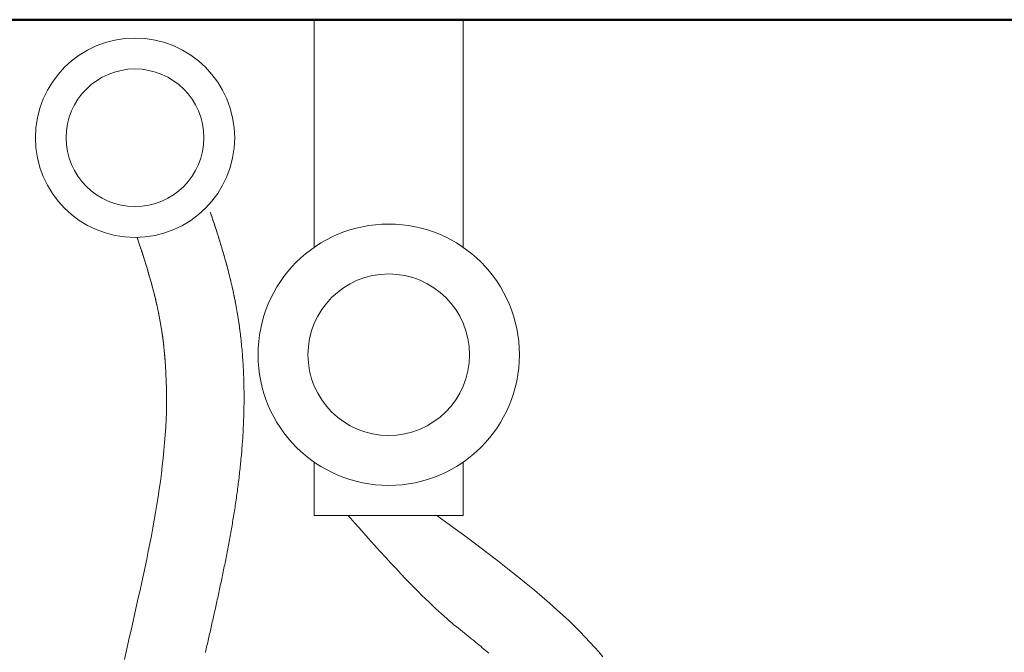
# Model space of a CAD drawing. Units: inches. Extents: x 64 to 1167, y 117 to 939.
# Tile 16 of 56: x 192.995 to 199.349, y 853.116 to 857.2. Entities that reach past the tile are written whole.
import ezdxf

# ---------------------------------------------------------------- set-up
doc = ezdxf.new("R2010")
doc.units = ezdxf.units.IN
doc.header["$MEASUREMENT"] = 0
doc.layers.add('A-FLOR-FIXT', color=8, linetype='Continuous', lineweight=18)
doc.layers.add('A-WALL', color=7, linetype='Continuous', lineweight=50)

# ---------------------------------------------------------------- blocks, each defined once
blk = doc.blocks.new('FAUCET')
for points in [[(1.4695, 2.7601), (0.0003, 2.7601), (0.0003, 1.7995), (1.4695, 1.7995)], [(2.8559, 1.7995), (3.2005, 1.7995), (3.2005, 2.7601), (2.8559, 2.7601)]]:
    blk.add_lwpolyline(points)
for points in [[(3.2005, 2.5912, 0), (3.2645, 2.6791, 0), (3.3257, 2.762, 0), (3.384, 2.8402, 0), (3.4397, 2.9138, 0), (3.493, 2.9831, 0), (3.5438, 3.0482, 0), (3.5924, 3.1094, 0), (3.639, 3.1668, 0), (3.6835, 3.2206, 0), (3.7262, 3.2711, 0), (3.7672, 3.3184, 0), (3.8067, 3.3628, 0), (3.8447, 3.4044, 0), (3.8814, 3.4435, 0), (3.9169, 3.4802, 0), (3.9514, 3.5148, 0), (3.985, 3.5473, 0), (4.0178, 3.5782, 0), (4.05, 3.6075, 0), (4.0816, 3.6354, 0), (4.1129, 3.6621, 0)], [(4.131, 0.5741, 0), (4.0812, 0.5853, 0), (4.0315, 0.5965, 0), (3.9816, 0.6078, 0), (3.9318, 0.6191, 0), (3.8819, 0.6304, 0), (3.8319, 0.6417, 0), (3.7819, 0.6529, 0), (3.7319, 0.6641, 0), (3.6819, 0.6752, 0), (3.6318, 0.6862, 0), (3.5817, 0.697, 0), (3.5316, 0.7077, 0), (3.4815, 0.7182, 0), (3.4313, 0.7284, 0), (3.3812, 0.7384, 0), (3.331, 0.7481, 0), (3.2809, 0.7575, 0), (3.2307, 0.7666, 0), (3.1806, 0.7753, 0), (3.1304, 0.7837, 0), (3.0803, 0.7916, 0), (3.0302, 0.7991, 0), (2.9801, 0.8062, 0), (2.93, 0.8128, 0), (2.88, 0.8188, 0), (2.83, 0.8244, 0), (2.78, 0.8293, 0), (2.73, 0.8337, 0), (2.6801, 0.8375, 0), (2.6302, 0.8406, 0), (2.5804, 0.8431, 0), (2.5307, 0.8449, 0), (2.4809, 0.846, 0), (2.4313, 0.8463, 0), (2.3817, 0.8458, 0), (2.3321, 0.8446, 0), (2.2827, 0.8426, 0), (2.2333, 0.8397, 0), (2.1839, 0.8359, 0), (2.1347, 0.8312, 0), (2.0855, 0.8256, 0), (2.0364, 0.8191, 0), (1.9874, 0.8116, 0), (1.9385, 0.8031, 0), (1.8897, 0.7936, 0), (1.8409, 0.7831, 0), (1.7923, 0.7717, 0), (1.7437, 0.7595, 0), (1.6952, 0.7465, 0), (1.6468, 0.7328, 0), (1.5984, 0.7185, 0), (1.55, 0.7035, 0), (1.5018, 0.6879, 0), (1.4535, 0.6719, 0), (1.4054, 0.6555, 0)], [(3.2005, 2.0185, 0), (3.2517, 2.0633, 0), (3.3003, 2.1062, 0), (3.3465, 2.1473, 0), (3.3904, 2.1866, 0), (3.4319, 2.2242, 0), (3.4713, 2.2602, 0), (3.5085, 2.2945, 0), (3.5437, 2.3273, 0), (3.5769, 2.3586, 0), (3.6083, 2.3884, 0), (3.6378, 2.4169, 0), (3.6656, 2.444, 0), (3.6917, 2.4699, 0), (3.7163, 2.4945, 0), (3.7394, 2.518, 0), (3.761, 2.5404, 0), (3.7814, 2.5617, 0), (3.8004, 2.582, 0), (3.8183, 2.6014, 0), (3.8351, 2.6199, 0), (3.8509, 2.6376, 0), (3.8657, 2.6545, 0), (3.8797, 2.6707, 0), (3.8929, 2.6862, 0), (3.9054, 2.7011, 0), (3.9172, 2.7154, 0), (3.9286, 2.7293, 0), (3.9394, 2.7427, 0), (3.9499, 2.7557, 0), (3.96, 2.7684, 0), (3.9699, 2.7808, 0), (3.9797, 2.7931, 0), (3.9893, 2.8051, 0), (3.9989, 2.8169, 0), (4.0083, 2.8285, 0), (4.0176, 2.84, 0), (4.0268, 2.8512, 0), (4.0359, 2.8623, 0), (4.0449, 2.8732, 0), (4.0538, 2.8839, 0), (4.0625, 2.8945, 0), (4.0712, 2.9048, 0), (4.0798, 2.9151, 0), (4.0883, 2.9251, 0)], [(4.0838, 1.0975, 0), (4.073, 1.0999, 0), (4.0622, 1.1023, 0), (4.0514, 1.1048, 0), (4.0406, 1.1072, 0), (4.0298, 1.1097, 0), (4.0189, 1.1121, 0), (4.0081, 1.1146, 0), (3.9972, 1.117, 0), (3.9863, 1.1195, 0), (3.9754, 1.1219, 0), (3.9645, 1.1244, 0), (3.9536, 1.1269, 0), (3.9426, 1.1293, 0), (3.9317, 1.1318, 0), (3.9207, 1.1342, 0), (3.9097, 1.1367, 0), (3.8988, 1.1392, 0), (3.8878, 1.1416, 0), (3.8767, 1.1441, 0), (3.8657, 1.1466, 0), (3.8547, 1.149, 0), (3.8437, 1.1515, 0), (3.8326, 1.154, 0), (3.8215, 1.1564, 0), (3.8104, 1.1589, 0), (3.7994, 1.1614, 0), (3.7883, 1.1638, 0), (3.7771, 1.1663, 0), (3.766, 1.1687, 0), (3.7549, 1.1712, 0), (3.7437, 1.1736, 0), (3.7325, 1.1761, 0), (3.7214, 1.1785, 0), (3.7102, 1.1809, 0), (3.699, 1.1834, 0), (3.6878, 1.1858, 0), (3.6765, 1.1882, 0), (3.6653, 1.1906, 0), (3.654, 1.193, 0), (3.6428, 1.1954, 0), (3.6315, 1.1978, 0), (3.6202, 1.2002, 0), (3.6089, 1.2026, 0), (3.5976, 1.205, 0), (3.5863, 1.2073, 0), (3.5749, 1.2097, 0), (3.5636, 1.212, 0), (3.5522, 1.2144, 0), (3.5409, 1.2167, 0), (3.5295, 1.219, 0), (3.5181, 1.2213, 0), (3.5067, 1.2236, 0), (3.4953, 1.2259, 0), (3.4838, 1.2282, 0), (3.4724, 1.2304, 0), (3.4609, 1.2327, 0), (3.4495, 1.2349, 0), (3.438, 1.2371, 0), (3.4265, 1.2394, 0), (3.415, 1.2416, 0), (3.4035, 1.2438, 0), (3.392, 1.2459, 0), (3.3804, 1.2481, 0), (3.3689, 1.2502, 0), (3.3573, 1.2524, 0), (3.3457, 1.2545, 0), (3.3342, 1.2566, 0), (3.3226, 1.2587, 0), (3.311, 1.2607, 0), (3.2993, 1.2628, 0), (3.2877, 1.2648, 0), (3.2761, 1.2669, 0), (3.2644, 1.2689, 0), (3.2527, 1.2708, 0), (3.2411, 1.2728, 0), (3.2294, 1.2748, 0), (3.2177, 1.2767, 0), (3.206, 1.2786, 0), (3.1942, 1.2805, 0), (3.1825, 1.2824, 0), (3.1708, 1.2842, 0), (3.159, 1.2861, 0), (3.1472, 1.2879, 0), (3.1354, 1.2897, 0), (3.1236, 1.2914, 0), (3.1118, 1.2932, 0), (3.1, 1.2949, 0), (3.0882, 1.2966, 0), (3.0764, 1.2983, 0), (3.0645, 1.2999, 0), (3.0526, 1.3016, 0), (3.0408, 1.3032, 0), (3.0289, 1.3048, 0), (3.017, 1.3063, 0), (3.0051, 1.3079, 0), (2.9932, 1.3094, 0), (2.9812, 1.3109, 0), (2.9693, 1.3123, 0), (2.9573, 1.3138, 0), (2.9454, 1.3152, 0), (2.9334, 1.3166, 0), (2.9214, 1.3179, 0), (2.9094, 1.3193, 0), (2.8974, 1.3206, 0), (2.8854, 1.3218, 0), (2.8733, 1.3231, 0), (2.8613, 1.3243, 0), (2.8492, 1.3255, 0), (2.8372, 1.3266, 0), (2.8251, 1.3278, 0), (2.813, 1.3289, 0), (2.8009, 1.3299, 0), (2.7888, 1.331, 0), (2.7767, 1.332, 0), (2.7645, 1.333, 0), (2.7524, 1.3339, 0), (2.7402, 1.3348, 0), (2.7281, 1.3357, 0), (2.7159, 1.3365, 0), (2.7037, 1.3374, 0), (2.6915, 1.3381, 0), (2.6793, 1.3389, 0), (2.6671, 1.3396, 0), (2.6548, 1.3403, 0), (2.6426, 1.3409, 0), (2.6303, 1.3415, 0), (2.6181, 1.3421, 0), (2.6058, 1.3427, 0), (2.5935, 1.3432, 0), (2.5812, 1.3436, 0), (2.5689, 1.3441, 0), (2.5566, 1.3445, 0), (2.5442, 1.3448, 0), (2.5319, 1.3451, 0), (2.5195, 1.3454, 0), (2.5072, 1.3457, 0), (2.4948, 1.3459, 0), (2.4824, 1.346, 0), (2.47, 1.3462, 0), (2.4576, 1.3462, 0), (2.4452, 1.3463, 0), (2.4328, 1.3463, 0), (2.4203, 1.3463, 0), (2.4079, 1.3462, 0), (2.3954, 1.3461, 0), (2.3829, 1.3459, 0), (2.3704, 1.3457, 0), (2.3579, 1.3455, 0), (2.3454, 1.3452, 0), (2.3329, 1.3449, 0), (2.3204, 1.3445, 0), (2.3079, 1.3441, 0), (2.2953, 1.3436, 0), (2.2828, 1.3431, 0), (2.2702, 1.3425, 0), (2.2576, 1.3419, 0), (2.2451, 1.3413, 0), (2.2325, 1.3406, 0), (2.2199, 1.3398, 0), (2.2073, 1.339, 0), (2.1946, 1.3382, 0), (2.182, 1.3373, 0), (2.1694, 1.3363, 0), (2.1567, 1.3354, 0), (2.1441, 1.3343, 0), (2.1314, 1.3332, 0), (2.1188, 1.3321, 0), (2.1061, 1.3309, 0), (2.0934, 1.3296, 0), (2.0807, 1.3283, 0), (2.068, 1.327, 0), (2.0553, 1.3255, 0), (2.0426, 1.3241, 0), (2.0299, 1.3226, 0), (2.0172, 1.321, 0), (2.0045, 1.3194, 0), (1.9917, 1.3177, 0), (1.979, 1.3159, 0), (1.9662, 1.3141, 0), (1.9535, 1.3123, 0), (1.9407, 1.3104, 0), (1.9279, 1.3084, 0), (1.9152, 1.3064, 0), (1.9024, 1.3043, 0), (1.8896, 1.3022, 0), (1.8769, 1.3, 0), (1.8642, 1.2977, 0), (1.8515, 1.2954, 0), (1.8388, 1.2931, 0), (1.8262, 1.2907, 0), (1.8136, 1.2882, 0), (1.801, 1.2857, 0), (1.7884, 1.2832, 0), (1.7759, 1.2806, 0), (1.7634, 1.2779, 0), (1.7509, 1.2752, 0), (1.7385, 1.2725, 0), (1.726, 1.2697, 0), (1.7137, 1.2669, 0), (1.7013, 1.264, 0), (1.689, 1.2611, 0), (1.6767, 1.2582, 0), (1.6644, 1.2552, 0), (1.6521, 1.2521, 0), (1.6399, 1.2491, 0), (1.6277, 1.246, 0), (1.6156, 1.2428, 0), (1.6034, 1.2396, 0), (1.5913, 1.2364, 0), (1.5792, 1.2332, 0), (1.5672, 1.2299, 0), (1.5552, 1.2266, 0), (1.5432, 1.2232, 0), (1.5312, 1.2199, 0), (1.5193, 1.2165, 0), (1.5074, 1.213, 0), (1.4955, 1.2096, 0), (1.4837, 1.2061, 0), (1.4719, 1.2026, 0), (1.4601, 1.199, 0), (1.4483, 1.1954, 0), (1.4366, 1.1919, 0), (1.4249, 1.1882, 0), (1.4133, 1.1846, 0), (1.4016, 1.181, 0), (1.39, 1.1773, 0), (1.3784, 1.1736, 0), (1.3669, 1.1699, 0), (1.3554, 1.1661, 0), (1.3439, 1.1624, 0), (1.3325, 1.1586, 0), (1.321, 1.1548, 0), (1.3097, 1.151, 0), (1.2983, 1.1472, 0), (1.287, 1.1434, 0), (1.2757, 1.1396, 0), (1.2644, 1.1357, 0), (1.2532, 1.1319, 0), (1.242, 1.128, 0)], [(2.0792, 1.3282, 0), (2.0747, 1.3277, 0), (2.0701, 1.3272, 0), (2.0655, 1.3267, 0), (2.0609, 1.3262, 0), (2.0563, 1.3257, 0), (2.0518, 1.3251, 0), (2.0472, 1.3246, 0), (2.0426, 1.3241, 0), (2.038, 1.3235, 0), (2.0334, 1.323, 0), (2.0288, 1.3224, 0), (2.0242, 1.3219, 0), (2.0197, 1.3213, 0), (2.0151, 1.3207, 0), (2.0105, 1.3201, 0), (2.0059, 1.3195, 0), (2.0013, 1.3189, 0), (1.9967, 1.3183, 0), (1.9921, 1.3177, 0), (1.9875, 1.3171, 0), (1.9829, 1.3165, 0), (1.9783, 1.3159, 0), (1.9737, 1.3152, 0), (1.9691, 1.3146, 0), (1.9645, 1.3139, 0), (1.9599, 1.3132, 0), (1.9553, 1.3126, 0), (1.9507, 1.3119, 0), (1.9461, 1.3112, 0), (1.9415, 1.3105, 0), (1.9369, 1.3098, 0), (1.9323, 1.3091, 0), (1.9277, 1.3084, 0), (1.9231, 1.3077, 0), (1.9185, 1.3069, 0), (1.9139, 1.3062, 0), (1.9093, 1.3054, 0), (1.9047, 1.3047, 0), (1.9001, 1.3039, 0), (1.8955, 1.3032, 0), (1.8909, 1.3024, 0), (1.8863, 1.3016, 0), (1.8817, 1.3008, 0), (1.8771, 1.3, 0), (1.8725, 1.2992, 0), (1.8679, 1.2984, 0), (1.8633, 1.2976, 0), (1.8587, 1.2968, 0), (1.8541, 1.2959, 0), (1.8496, 1.2951, 0), (1.845, 1.2943, 0), (1.8404, 1.2934, 0), (1.8359, 1.2925, 0), (1.8313, 1.2917, 0), (1.8268, 1.2908, 0), (1.8222, 1.2899, 0), (1.8177, 1.289, 0), (1.8131, 1.2882, 0), (1.8086, 1.2873, 0), (1.804, 1.2863, 0), (1.7995, 1.2854, 0), (1.795, 1.2845, 0), (1.7904, 1.2836, 0), (1.7859, 1.2827, 0), (1.7814, 1.2817, 0), (1.7769, 1.2808, 0), (1.7724, 1.2798, 0), (1.7679, 1.2789, 0), (1.7634, 1.2779, 0), (1.7589, 1.277, 0), (1.7544, 1.276, 0), (1.7499, 1.275, 0), (1.7454, 1.274, 0), (1.7409, 1.273, 0), (1.7364, 1.272, 0), (1.7319, 1.271, 0), (1.7275, 1.27, 0), (1.723, 1.269, 0), (1.7185, 1.268, 0), (1.714, 1.267, 0), (1.7096, 1.266, 0), (1.7051, 1.2649, 0), (1.7007, 1.2639, 0), (1.6962, 1.2628, 0), (1.6918, 1.2618, 0), (1.6873, 1.2607, 0), (1.6829, 1.2597, 0), (1.6785, 1.2586, 0), (1.674, 1.2575, 0), (1.6696, 1.2564, 0), (1.6652, 1.2554, 0), (1.6607, 1.2543, 0), (1.6563, 1.2532, 0), (1.6519, 1.2521, 0), (1.6475, 1.251, 0), (1.6431, 1.2499, 0), (1.6387, 1.2488, 0), (1.6343, 1.2476, 0), (1.6299, 1.2465, 0), (1.6255, 1.2454, 0), (1.6211, 1.2443, 0), (1.6167, 1.2431, 0), (1.6124, 1.242, 0), (1.608, 1.2408, 0), (1.6036, 1.2397, 0), (1.5992, 1.2385, 0), (1.5949, 1.2374, 0), (1.5905, 1.2362, 0), (1.5862, 1.235, 0), (1.5818, 1.2339, 0), (1.5774, 1.2327, 0), (1.5731, 1.2315, 0), (1.5688, 1.2303, 0), (1.5644, 1.2291, 0), (1.5601, 1.2279, 0), (1.5558, 1.2267, 0), (1.5514, 1.2255, 0), (1.5471, 1.2243, 0), (1.5428, 1.2231, 0), (1.5385, 1.2219, 0), (1.5342, 1.2207, 0), (1.5298, 1.2195, 0), (1.5255, 1.2182, 0), (1.5212, 1.217, 0), (1.5169, 1.2158, 0), (1.5126, 1.2145, 0), (1.5084, 1.2133, 0), (1.5041, 1.2121, 0), (1.4998, 1.2108, 0), (1.4955, 1.2096, 0), (1.4912, 1.2083, 0), (1.487, 1.207, 0), (1.4827, 1.2058, 0), (1.4784, 1.2045, 0), (1.4742, 1.2032, 0), (1.4699, 1.202, 0), (1.4657, 1.2007, 0), (1.4614, 1.1994, 0), (1.4572, 1.1981, 0), (1.4529, 1.1969, 0), (1.4487, 1.1956, 0), (1.4445, 1.1943, 0), (1.4403, 1.193, 0), (1.436, 1.1917, 0), (1.4318, 1.1904, 0), (1.4276, 1.1891, 0), (1.4234, 1.1878, 0), (1.4192, 1.1865, 0), (1.415, 1.1851, 0), (1.4108, 1.1838, 0), (1.4066, 1.1825, 0), (1.4024, 1.1812, 0), (1.3982, 1.1799, 0), (1.394, 1.1785, 0), (1.3898, 1.1772, 0), (1.3856, 1.1759, 0), (1.3815, 1.1746, 0), (1.3773, 1.1732, 0), (1.3731, 1.1719, 0), (1.369, 1.1705, 0), (1.3648, 1.1692, 0), (1.3607, 1.1678, 0), (1.3565, 1.1665, 0), (1.3524, 1.1652, 0), (1.3482, 1.1638, 0), (1.3441, 1.1624, 0), (1.34, 1.1611, 0), (1.3358, 1.1597, 0), (1.3317, 1.1584, 0), (1.3276, 1.157, 0), (1.3235, 1.1556, 0), (1.3194, 1.1543, 0), (1.3153, 1.1529, 0), (1.3112, 1.1515, 0), (1.307, 1.1502, 0), (1.303, 1.1488, 0), (1.2989, 1.1474, 0), (1.2948, 1.146, 0), (1.2907, 1.1447, 0), (1.2866, 1.1433, 0), (1.2825, 1.1419, 0), (1.2785, 1.1405, 0), (1.2744, 1.1391, 0), (1.2703, 1.1378, 0), (1.2663, 1.1364, 0), (1.2622, 1.135, 0), (1.2582, 1.1336, 0), (1.2541, 1.1322, 0), (1.2501, 1.1308, 0), (1.246, 1.1294, 0), (1.242, 1.128, 0)], [(2.2006, 0.8373, 0), (2.1956, 0.8369, 0), (2.1905, 0.8364, 0), (2.1854, 0.836, 0), (2.1804, 0.8356, 0), (2.1753, 0.8351, 0), (2.1702, 0.8347, 0), (2.1652, 0.8342, 0), (2.1601, 0.8337, 0), (2.155, 0.8333, 0), (2.15, 0.8328, 0), (2.1449, 0.8323, 0), (2.1399, 0.8318, 0), (2.1348, 0.8312, 0), (2.1298, 0.8307, 0), (2.1247, 0.8302, 0), (2.1196, 0.8296, 0), (2.1146, 0.8291, 0), (2.1095, 0.8285, 0), (2.1045, 0.8279, 0), (2.0994, 0.8273, 0), (2.0944, 0.8267, 0), (2.0893, 0.8261, 0), (2.0843, 0.8255, 0), (2.0792, 0.8249, 0), (2.0742, 0.8242, 0), (2.0691, 0.8236, 0), (2.0641, 0.8229, 0), (2.059, 0.8222, 0), (2.054, 0.8216, 0), (2.049, 0.8209, 0), (2.0439, 0.8202, 0), (2.0389, 0.8194, 0), (2.0338, 0.8187, 0), (2.0288, 0.818, 0), (2.0238, 0.8173, 0), (2.0187, 0.8165, 0), (2.0137, 0.8157, 0), (2.0087, 0.815, 0), (2.0036, 0.8142, 0), (1.9986, 0.8134, 0), (1.9936, 0.8126, 0), (1.9885, 0.8118, 0), (1.9835, 0.8109, 0), (1.9785, 0.8101, 0), (1.9734, 0.8093, 0), (1.9684, 0.8084, 0), (1.9634, 0.8075, 0), (1.9583, 0.8067, 0), (1.9533, 0.8058, 0), (1.9483, 0.8049, 0), (1.9433, 0.8039, 0), (1.9383, 0.803, 0), (1.9332, 0.8021, 0), (1.9282, 0.8012, 0), (1.9232, 0.8002, 0), (1.9182, 0.7992, 0), (1.9132, 0.7983, 0), (1.9081, 0.7973, 0), (1.9031, 0.7963, 0), (1.8981, 0.7953, 0), (1.8931, 0.7943, 0), (1.8881, 0.7932, 0), (1.8831, 0.7922, 0), (1.8781, 0.7911, 0), (1.8731, 0.7901, 0), (1.868, 0.789, 0), (1.863, 0.788, 0), (1.858, 0.7869, 0), (1.853, 0.7858, 0), (1.848, 0.7847, 0), (1.843, 0.7836, 0), (1.838, 0.7824, 0), (1.833, 0.7813, 0), (1.828, 0.7802, 0), (1.823, 0.779, 0), (1.818, 0.7778, 0), (1.813, 0.7767, 0), (1.808, 0.7755, 0), (1.803, 0.7743, 0), (1.798, 0.7731, 0), (1.793, 0.7719, 0), (1.788, 0.7707, 0), (1.783, 0.7695, 0), (1.778, 0.7682, 0), (1.773, 0.767, 0), (1.768, 0.7657, 0), (1.7631, 0.7645, 0), (1.7581, 0.7632, 0), (1.7531, 0.7619, 0), (1.7481, 0.7607, 0), (1.7431, 0.7594, 0), (1.7381, 0.7581, 0), (1.7331, 0.7568, 0), (1.7281, 0.7554, 0), (1.7232, 0.7541, 0), (1.7182, 0.7528, 0), (1.7132, 0.7514, 0), (1.7082, 0.7501, 0), (1.7032, 0.7487, 0), (1.6982, 0.7474, 0), (1.6933, 0.746, 0), (1.6883, 0.7446, 0), (1.6833, 0.7432, 0), (1.6783, 0.7418, 0), (1.6733, 0.7404, 0), (1.6684, 0.739, 0), (1.6634, 0.7376, 0), (1.6584, 0.7362, 0), (1.6534, 0.7348, 0), (1.6485, 0.7333, 0), (1.6435, 0.7319, 0), (1.6385, 0.7304, 0), (1.6335, 0.729, 0), (1.6286, 0.7275, 0), (1.6236, 0.726, 0), (1.6186, 0.7245, 0), (1.6136, 0.7231, 0), (1.6087, 0.7216, 0), (1.6037, 0.7201, 0), (1.5987, 0.7186, 0), (1.5938, 0.7171, 0), (1.5888, 0.7155, 0), (1.5838, 0.714, 0), (1.5789, 0.7125, 0), (1.5739, 0.7109, 0), (1.5689, 0.7094, 0), (1.564, 0.7078, 0), (1.559, 0.7063, 0), (1.554, 0.7047, 0), (1.5491, 0.7032, 0), (1.5441, 0.7016, 0), (1.5392, 0.7, 0), (1.5342, 0.6984, 0), (1.5292, 0.6968, 0), (1.5243, 0.6952, 0), (1.5193, 0.6936, 0), (1.5144, 0.692, 0), (1.5094, 0.6904, 0), (1.5044, 0.6888, 0), (1.4995, 0.6872, 0), (1.4945, 0.6856, 0), (1.4896, 0.6839, 0), (1.4846, 0.6823, 0), (1.4796, 0.6807, 0), (1.4747, 0.679, 0), (1.4697, 0.6774, 0), (1.4648, 0.6757, 0), (1.4598, 0.674, 0), (1.4549, 0.6724, 0), (1.4499, 0.6707, 0), (1.445, 0.669, 0), (1.44, 0.6673, 0), (1.4351, 0.6657, 0), (1.4301, 0.664, 0), (1.4252, 0.6623, 0), (1.4202, 0.6606, 0), (1.4153, 0.6589, 0), (1.4103, 0.6572, 0), (1.4054, 0.6555, 0)], [(2.2006, 0.8373, 0), (2.1956, 0.8369, 0), (2.1905, 0.8364, 0), (2.1854, 0.836, 0), (2.1804, 0.8356, 0), (2.1753, 0.8351, 0), (2.1702, 0.8347, 0), (2.1652, 0.8342, 0), (2.1601, 0.8337, 0), (2.155, 0.8333, 0), (2.15, 0.8328, 0), (2.1449, 0.8323, 0), (2.1399, 0.8318, 0), (2.1348, 0.8312, 0), (2.1298, 0.8307, 0), (2.1247, 0.8302, 0), (2.1196, 0.8296, 0), (2.1146, 0.8291, 0), (2.1095, 0.8285, 0), (2.1045, 0.8279, 0), (2.0994, 0.8273, 0), (2.0944, 0.8267, 0), (2.0893, 0.8261, 0), (2.0843, 0.8255, 0), (2.0792, 0.8249, 0), (2.0742, 0.8242, 0), (2.0691, 0.8236, 0), (2.0641, 0.8229, 0), (2.059, 0.8222, 0), (2.054, 0.8216, 0), (2.049, 0.8209, 0), (2.0439, 0.8202, 0), (2.0389, 0.8194, 0), (2.0338, 0.8187, 0), (2.0288, 0.818, 0), (2.0238, 0.8173, 0), (2.0187, 0.8165, 0), (2.0137, 0.8157, 0), (2.0087, 0.815, 0), (2.0036, 0.8142, 0), (1.9986, 0.8134, 0), (1.9936, 0.8126, 0), (1.9885, 0.8118, 0), (1.9835, 0.8109, 0), (1.9785, 0.8101, 0), (1.9734, 0.8093, 0), (1.9684, 0.8084, 0), (1.9634, 0.8075, 0), (1.9583, 0.8067, 0), (1.9533, 0.8058, 0), (1.9483, 0.8049, 0), (1.9433, 0.8039, 0), (1.9383, 0.803, 0), (1.9332, 0.8021, 0), (1.9282, 0.8012, 0), (1.9232, 0.8002, 0), (1.9182, 0.7992, 0), (1.9132, 0.7983, 0), (1.9081, 0.7973, 0), (1.9031, 0.7963, 0), (1.8981, 0.7953, 0), (1.8931, 0.7943, 0), (1.8881, 0.7932, 0), (1.8831, 0.7922, 0), (1.8781, 0.7911, 0), (1.8731, 0.7901, 0), (1.868, 0.789, 0), (1.863, 0.788, 0), (1.858, 0.7869, 0), (1.853, 0.7858, 0), (1.848, 0.7847, 0), (1.843, 0.7836, 0), (1.838, 0.7824, 0), (1.833, 0.7813, 0), (1.828, 0.7802, 0), (1.823, 0.779, 0), (1.818, 0.7778, 0), (1.813, 0.7767, 0), (1.808, 0.7755, 0), (1.803, 0.7743, 0), (1.798, 0.7731, 0), (1.793, 0.7719, 0), (1.788, 0.7707, 0), (1.783, 0.7695, 0), (1.778, 0.7682, 0), (1.773, 0.767, 0), (1.768, 0.7657, 0), (1.7631, 0.7645, 0), (1.7581, 0.7632, 0), (1.7531, 0.7619, 0), (1.7481, 0.7607, 0), (1.7431, 0.7594, 0), (1.7381, 0.7581, 0), (1.7331, 0.7568, 0), (1.7281, 0.7554, 0), (1.7232, 0.7541, 0), (1.7182, 0.7528, 0), (1.7132, 0.7514, 0), (1.7082, 0.7501, 0), (1.7032, 0.7487, 0), (1.6982, 0.7474, 0), (1.6933, 0.746, 0), (1.6883, 0.7446, 0), (1.6833, 0.7432, 0), (1.6783, 0.7418, 0), (1.6733, 0.7404, 0), (1.6684, 0.739, 0), (1.6634, 0.7376, 0), (1.6584, 0.7362, 0), (1.6534, 0.7348, 0), (1.6485, 0.7333, 0), (1.6435, 0.7319, 0), (1.6385, 0.7304, 0), (1.6335, 0.729, 0), (1.6286, 0.7275, 0), (1.6236, 0.726, 0), (1.6186, 0.7245, 0), (1.6136, 0.7231, 0), (1.6087, 0.7216, 0), (1.6037, 0.7201, 0), (1.5987, 0.7186, 0), (1.5938, 0.7171, 0), (1.5888, 0.7155, 0), (1.5838, 0.714, 0), (1.5789, 0.7125, 0), (1.5739, 0.7109, 0), (1.5689, 0.7094, 0), (1.564, 0.7078, 0), (1.559, 0.7063, 0), (1.554, 0.7047, 0), (1.5491, 0.7032, 0), (1.5441, 0.7016, 0), (1.5392, 0.7, 0), (1.5342, 0.6984, 0), (1.5292, 0.6968, 0), (1.5243, 0.6952, 0), (1.5193, 0.6936, 0), (1.5144, 0.692, 0), (1.5094, 0.6904, 0), (1.5044, 0.6888, 0), (1.4995, 0.6872, 0), (1.4945, 0.6856, 0), (1.4896, 0.6839, 0), (1.4846, 0.6823, 0), (1.4796, 0.6807, 0), (1.4747, 0.679, 0), (1.4697, 0.6774, 0), (1.4648, 0.6757, 0), (1.4598, 0.674, 0), (1.4549, 0.6724, 0), (1.4499, 0.6707, 0), (1.445, 0.669, 0), (1.44, 0.6673, 0), (1.4351, 0.6657, 0), (1.4301, 0.664, 0), (1.4252, 0.6623, 0), (1.4202, 0.6606, 0), (1.4153, 0.6589, 0), (1.4103, 0.6572, 0), (1.4054, 0.6555, 0)]]:
    blk.add_polyline3d(points)
for centre, radius in [((2.1627, 2.2798), 0.8433), ((2.1627, 2.2798), 0.5212), ((0.7624, 0.6428), 0.6431), ((0.7624, 0.6428), 0.4442)]:
    blk.add_circle(centre, radius)

msp = doc.modelspace()

# ---------------------------------------------------------------- linework, layer by layer
at = {"layer": 'A-WALL'}
msp.add_line((297.1073, 857.1998), (183.1073, 857.1998), dxfattribs=at)

# ---------------------------------------------------------------- block references
at = {"layer": 'A-FLOR-FIXT', "rotation": 270.0000000000299}
msp.add_blockref('FAUCET', (193.0969, 857.2), dxfattribs=at)

doc.saveas('drawing.dxf')
